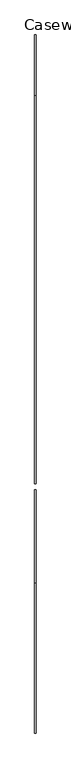
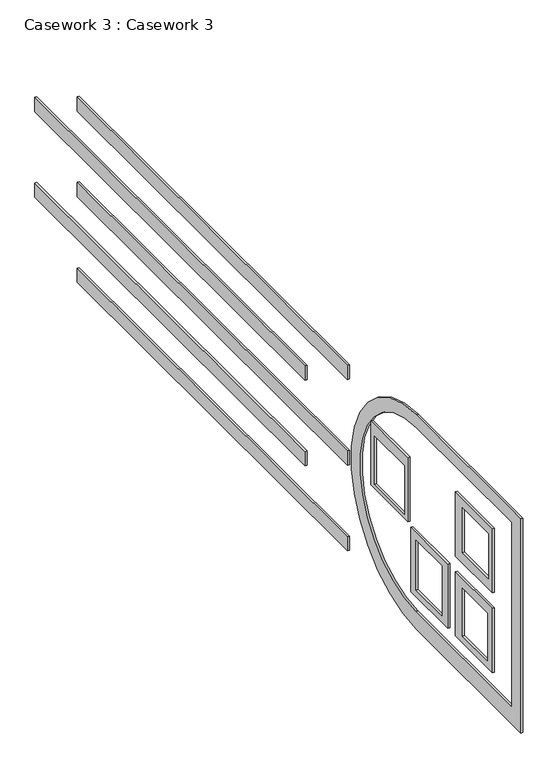
"""IFC4 building model written with IfcOpenShell, lengths in millimetres: furniture geometry, Casework 3 : Casework 3."""

from ifc_helpers import new_model, si_unit, point, frame, frame_2d, origin, place, context, project, spatial, polyline, circle_curve, trimmed, segment, composite_curve, outline, extrude, source, transform, mapped, element, save


def casework_3_casework_3_5667240a(model_context):
    return source(origin(), model_context, "Body", "SweptSolid", [
        extrude(outline(composite_curve([segment(polyline([(747.0423438, 3410.9248695), (3185.4423438, 3410.9248695)]), True, "CONTINUOUS"), segment(trimmed(circle_curve(frame_2d((3185.4423438, 1886.9248695)), 1524.0), [point((3185.4423438, 3410.9248695))], [point((3185.4423438, 362.9248695))], False, "CARTESIAN"), True, "CONTINUOUS"), segment(polyline([(3185.4423438, 362.9248695), (747.0423438, 362.9248695), (747.0423438, 3410.9248695)]), True, "CONTINUOUS")], self_intersect=False), holes=[composite_curve([segment(polyline([(970.4257925, 609.6), (3192.9257925, 609.6)]), True, "CONTINUOUS"), segment(trimmed(circle_curve(frame_2d((3192.9257925, 1917.7)), 1308.1), [point((3192.9257925, 609.6))], [point((3192.9257925, 3225.8))], True, "CARTESIAN"), True, "CONTINUOUS"), segment(polyline([(3192.9257925, 3225.8), (970.4257925, 3225.8), (970.4257925, 609.6)]), True, "CONTINUOUS")], self_intersect=False)]), frame((2684.6501403, 0.0, 0.0), z_axis=(1.0, 0.0, 0.0), x_axis=(0.0, 1.0, 0.0)), (0.0, 0.0, 1.0), 25.4),
        extrude(outline(polyline([(2274.7912653, 2868.8216932), (2274.7912653, 1954.4216932), (1411.1912653, 1954.4216932), (1411.1912653, 2868.8216932), (2274.7912653, 2868.8216932)]), holes=[polyline([(2113.4257925, 2743.2), (1503.8257925, 2743.2), (1503.8257925, 2101.85), (2113.4257925, 2101.85), (2113.4257925, 2743.2)])]), frame((2684.6501403, 0.0, 0.0), z_axis=(1.0, 0.0, 0.0), x_axis=(0.0, 1.0, 0.0)), (0.0, 0.0, 1.0), 25.4),
        extrude(outline(polyline([(2274.7912653, 1733.55), (2274.7912653, 819.15), (1411.1912653, 819.15), (1411.1912653, 1733.55), (2274.7912653, 1733.55)]), holes=[polyline([(2113.4257925, 1593.85), (1529.2257925, 1593.85), (1529.2257925, 914.4), (2113.4257925, 914.4), (2113.4257925, 1593.85)])]), frame((2684.6501403, 0.0, 0.0), z_axis=(1.0, 0.0, 0.0), x_axis=(0.0, 1.0, 0.0)), (0.0, 0.0, 1.0), 25.4),
        extrude(outline(polyline([(3316.1912653, 1733.55), (3316.1912653, 819.15), (2452.5912653, 819.15), (2452.5912653, 1733.55), (3316.1912653, 1733.55)]), holes=[polyline([(3192.9257925, 1625.6), (2586.5007925, 1625.6), (2586.5007925, 914.4), (3192.9257925, 914.4), (3192.9257925, 1625.6)])]), frame((2684.6501403, 0.0, 0.0), z_axis=(1.0, 0.0, 0.0), x_axis=(0.0, 1.0, 0.0)), (0.0, 0.0, 1.0), 25.4),
        extrude(outline(polyline([(4248.9126398, 2683.4804792), (4248.9126398, 1769.0804792), (3385.3126398, 1769.0804792), (3385.3126398, 2683.4804792), (4248.9126398, 2683.4804792)]), holes=[polyline([(4164.6184081, 2514.6), (3465.6606931, 2514.6), (3465.6606931, 1828.8), (4164.6184081, 1828.8), (4164.6184081, 2514.6)])]), frame((2684.6501403, 0.0, 0.0), z_axis=(1.0, 0.0, 0.0), x_axis=(0.0, 1.0, 0.0)), (0.0, 0.0, 1.0), 25.4),
        extrude(outline(polyline([(2710.0501403, 11094.9163997), (2710.0501403, 4795.7163997), (2684.6501403, 4795.7163997), (2684.6501403, 11094.9163997), (2710.0501403, 11094.9163997)])), frame((0.0, 0.0, 2937.4804792), z_axis=(0.0, 0.0, 1.0), x_axis=(1.0, 0.0, 0.0)), (0.0, 0.0, 1.0), 203.2),
        extrude(outline(polyline([(2710.0501403, 12085.5163997), (2710.0501403, 5786.3163997), (2684.6501403, 5786.3163997), (2684.6501403, 12085.5163997), (2710.0501403, 12085.5163997)])), frame((0.0, 0.0, 2327.8804792), z_axis=(0.0, 0.0, 1.0), x_axis=(1.0, 0.0, 0.0)), (0.0, 0.0, 1.0), 203.2),
        extrude(outline(polyline([(2710.0501403, 11094.9163997), (2710.0501403, 4795.7163997), (2684.6501403, 4795.7163997), (2684.6501403, 11094.9163997), (2710.0501403, 11094.9163997)])), frame((0.0, 0.0, 1718.2804792), z_axis=(0.0, 0.0, 1.0), x_axis=(1.0, 0.0, 0.0)), (0.0, 0.0, 1.0), 203.2),
        extrude(outline(polyline([(2710.0501403, 12085.5163997), (2710.0501403, 5786.3163997), (2684.6501403, 5786.3163997), (2684.6501403, 12085.5163997), (2710.0501403, 12085.5163997)])), frame((0.0, 0.0, 1108.6804792), z_axis=(0.0, 0.0, 1.0), x_axis=(1.0, 0.0, 0.0)), (0.0, 0.0, 1.0), 203.2),
        extrude(outline(polyline([(2710.0501403, 11094.9163997), (2710.0501403, 4795.7163997), (2684.6501403, 4795.7163997), (2684.6501403, 11094.9163997), (2710.0501403, 11094.9163997)])), frame((0.0, 0.0, 499.0804792), z_axis=(0.0, 0.0, 1.0), x_axis=(1.0, 0.0, 0.0)), (0.0, 0.0, 1.0), 203.2),
    ])


if __name__ == "__main__":
    model = new_model("IFC4")
    model_context = context("Model", 3, world=origin())
    ifc_project = project(units=[si_unit("LENGTHUNIT", "METRE", prefix="MILLI")], contexts=[model_context])
    site = spatial("IfcSite", under=ifc_project)
    building = spatial("IfcBuilding", under=site)
    placement = place(None, origin())
    casework_3_casework_3_shape = casework_3_casework_3_5667240a(model_context)
    element("IfcFurniture", 1, ObjectType="Casework 3 : Casework 3", at=placement, inside=building, context=model_context, shape_type="MappedRepresentation", body=[
        mapped(casework_3_casework_3_shape, transform((0.0, 0.0, 0.0), x_axis=(1.0, 0.0, 0.0), y_axis=(0.0, 1.0, 0.0), z_axis=(0.0, 0.0, 1.0))),
    ])
    save(model, "model.ifc")

# Revit data of these elements
# Element 1 (IfcFurniture, "Casework 3 : Casework 3")
#   Materials on its faces: "Laminate, Ivory, Matte"
# Materials
#   "Laminate, Ivory, Matte": class "Plastic", colour RGB 247 247 239, transparency 0, Description = "Plastic Laminate - Ivory, Matte", Cost = 0
